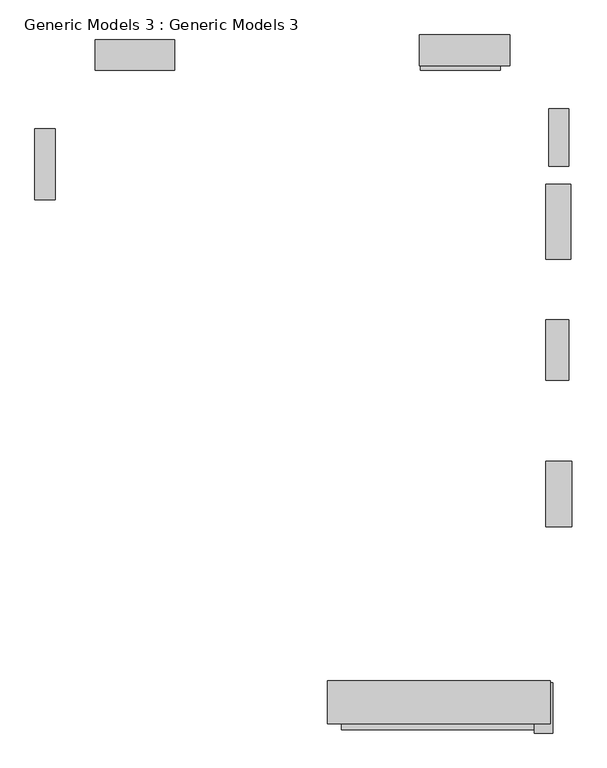
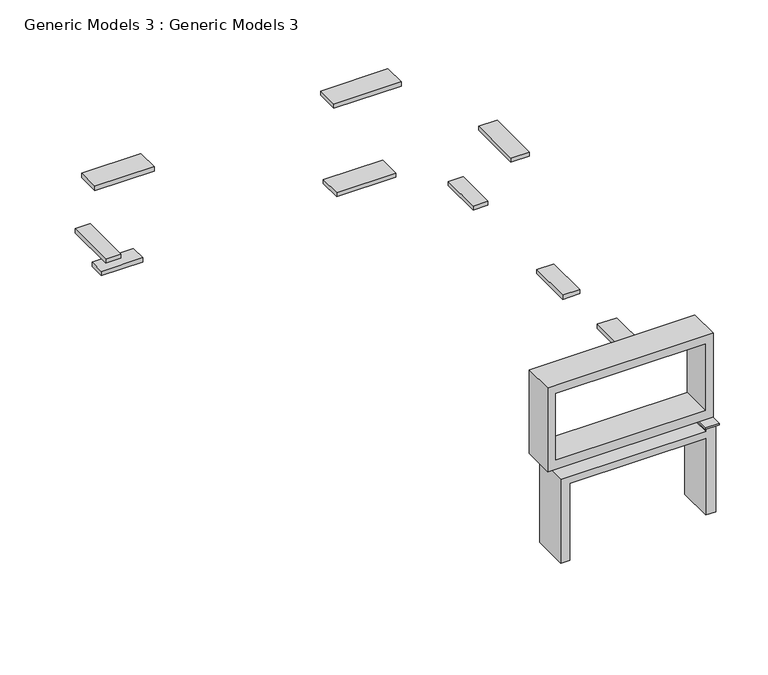
"""IFC4 building model written with IfcOpenShell, lengths in millimetres: proxy geometry, Generic Models 3 : Generic Models 3."""

from ifc_helpers import new_model, si_unit, frame, origin, place, context, project, spatial, polyline, outline, extrude, source, transform, mapped, element, save


def generic_models_3_generic_models_3_41235341(model_context):
    return source(origin(), model_context, "Body", "SweptSolid", [
        extrude(outline(polyline([(-23986.2386697, 1886.9888122), (-23465.5386697, 1886.9888122), (-23465.5386697, 73.8617848), (-23986.2386697, 73.8617848), (-23986.2386697, 1886.9888122)])), frame((0.0, 0.0, 5453.2250414), z_axis=(0.0, 0.0, 1.0), x_axis=(1.0, 0.0, 0.0)), (0.0, 0.0, 1.0), 152.4),
        extrude(outline(polyline([(-22161.002576, 3492.5488046), (-22161.002576, 4041.9318871), (-20738.602576, 4041.9318871), (-20738.602576, 3492.5488046), (-22161.002576, 3492.5488046)])), frame((0.0, 0.0, 2287.6988382), z_axis=(0.0, 0.0, 1.0), x_axis=(1.0, 0.0, 0.0)), (0.0, 0.0, 1.0), 152.4),
        extrude(outline(polyline([(-22441.7106462, 3378.2488046), (-22441.7106462, 4161.7100099), (-20411.1886697, 4161.7100099), (-20411.1886697, 3378.2488046), (-22441.7106462, 3378.2488046)])), frame((0.0, 0.0, 5548.8556249), z_axis=(0.0, 0.0, 1.0), x_axis=(1.0, 0.0, 0.0)), (0.0, 0.0, 1.0), 152.4),
        extrude(outline(polyline([(-14136.7349532, 3378.2488046), (-14136.7349532, 4161.7100099), (-12099.0386697, 4161.7100099), (-12099.0386697, 3378.2488046), (-14136.7349532, 3378.2488046)])), frame((0.0, 0.0, 2411.6935747), z_axis=(0.0, 0.0, 1.0), x_axis=(1.0, 0.0, 0.0)), (0.0, 0.0, 1.0), 152.4),
        extrude(outline(polyline([(-14160.3753926, 3492.5488046), (-14160.3753926, 4280.2702798), (-11848.9753926, 4280.2702798), (-11848.9753926, 3492.5488046), (-14160.3753926, 3492.5488046)])), frame((0.0, 0.0, 5569.0204449), z_axis=(0.0, 0.0, 1.0), x_axis=(1.0, 0.0, 0.0)), (0.0, 0.0, 1.0), 152.4),
        extrude(outline(polyline([(-10346.4386697, 927.1488046), (-10857.170432, 927.1488046), (-10857.170432, 2394.3257833), (-10346.4386697, 2394.3257833), (-10346.4386697, 927.1488046)])), frame((0.0, 0.0, 2267.0732017), z_axis=(0.0, 0.0, 1.0), x_axis=(1.0, 0.0, 0.0)), (0.0, 0.0, 1.0), 152.4),
        extrude(outline(polyline([(-10295.6386697, -1441.4011954), (-10930.6386697, -1441.4011954), (-10930.6386697, 469.9488046), (-10295.6386697, 469.9488046), (-10295.6386697, -1441.4011954)])), frame((0.0, 0.0, 5470.7760363), z_axis=(0.0, 0.0, 1.0), x_axis=(1.0, 0.0, 0.0)), (0.0, 0.0, 1.0), 152.4),
        extrude(outline(polyline([(-10346.4386697, -4526.8642074), (-10930.6386697, -4526.8642074), (-10930.6386697, -2990.8011954), (-10346.4386697, -2990.8011954), (-10346.4386697, -4526.8642074)])), frame((0.0, 0.0, 2353.4996799), z_axis=(0.0, 0.0, 1.0), x_axis=(1.0, 0.0, 0.0)), (0.0, 0.0, 1.0), 152.4),
        extrude(outline(polyline([(-10270.2386697, -8271.2002822), (-10930.6386697, -8271.2002822), (-10930.6386697, -6603.9511954), (-10270.2386697, -6603.9511954), (-10270.2386697, -8271.2002822)])), frame((0.0, 0.0, 2556.4176523), z_axis=(0.0, 0.0, 1.0), x_axis=(1.0, 0.0, 0.0)), (0.0, 0.0, 1.0), 152.4),
        extrude(outline(polyline([(6400.8, -10816.3386697), (6400.8, -16512.2886697), (3352.8, -16512.2886697), (3352.8, -10816.3386697), (6400.8, -10816.3386697)]), holes=[polyline([(6096.0, -11084.1908348), (3684.4190385, -11084.1908348), (3684.4190385, -16224.7214825), (6096.0, -16224.7214825), (6096.0, -11084.1908348)])]), frame((0.0, -13298.425338, 0.0), z_axis=(0.0, 1.0, 0.0), x_axis=(0.0, 0.0, 1.0)), (0.0, 0.0, 1.0), 1093.7741426),
        extrude(outline(polyline([(-11229.0886697, -12255.4511954), (-10751.7286468, -12255.4511954), (-10751.7286468, -13538.1511954), (-11229.0886697, -13538.1511954), (-11229.0886697, -12255.4511954)])), frame((0.0, 0.0, 3187.4397174), z_axis=(0.0, 0.0, 1.0), x_axis=(1.0, 0.0, 0.0)), (0.0, 0.0, 1.0), 50.8),
        extrude(outline(polyline([(0.0, -16150.3386697), (0.0, -15845.5386697), (2790.1948734, -15845.5386697), (2790.1948734, -11164.2034433), (0.0, -11164.2034433), (0.0, -10816.3386697), (3187.4397174, -10816.3386697), (3187.4397174, -11164.2034433), (3048.0, -11164.2034433), (3048.0, -16150.3386697), (0.0, -16150.3386697)])), frame((0.0, -13454.2956142, 0.0), z_axis=(0.0, 1.0, 0.0), x_axis=(0.0, 0.0, 1.0)), (0.0, 0.0, 1.0), 1249.6444188),
    ])


if __name__ == "__main__":
    model = new_model("IFC4")
    model_context = context("Model", 3, world=origin())
    ifc_project = project(units=[si_unit("LENGTHUNIT", "METRE", prefix="MILLI")], contexts=[model_context])
    site = spatial("IfcSite", under=ifc_project)
    building = spatial("IfcBuilding", under=site)
    placement = place(None, origin())
    generic_models_3_generic_models_3_shape = generic_models_3_generic_models_3_41235341(model_context)
    element("IfcBuildingElementProxy", 1, Name="Generic Models 3 : Generic Models 3", ObjectType="Generic Models 3 : Generic Models 3", at=placement, inside=building, context=model_context, shape_type="MappedRepresentation", body=[
        mapped(generic_models_3_generic_models_3_shape, transform((0.0, 0.0, 0.0), x_axis=(1.0, 0.0, 0.0), y_axis=(0.0, 1.0, 0.0), z_axis=(0.0, 0.0, 1.0))),
    ])
    save(model, "model.ifc")
